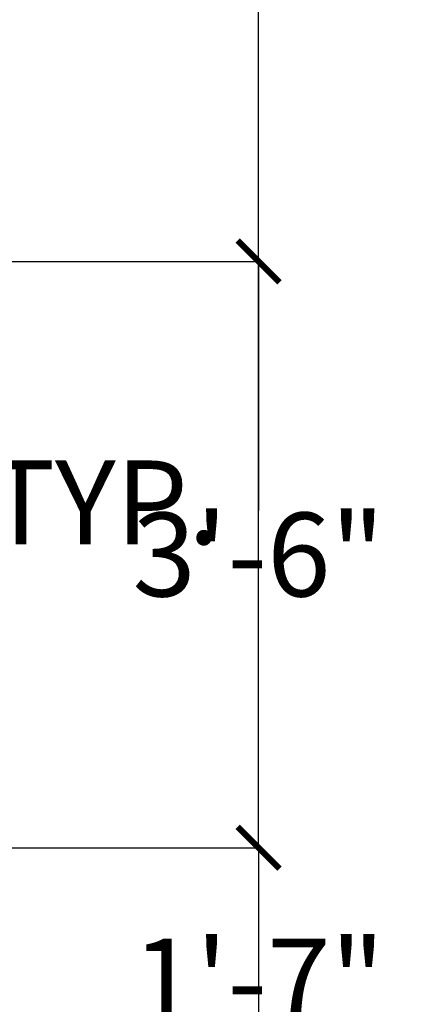
# Model space of a CAD drawing. Units: inches. Extents: x 2278 to 7495, y -71 to 1198.
# Tile 36 of 44: x 5150 to 5179, y 107 to 178. Entities that reach past the tile are written whole.
import ezdxf

# ---------------------------------------------------------------- set-up
doc = ezdxf.new("R2010")
doc.units = ezdxf.units.IN
doc.header["$MEASUREMENT"] = 0
doc.layers.add('A-ANNO-DIMS', color=2, linetype='Continuous', lineweight=18)
doc.styles.get("Standard").update_dxf_attribs({"font": 'arial.ttf'})
doc.dimstyles.get("Standard").update_dxf_attribs({"dimtxt": 6, "dimasz": 3, "dimexe": 0.18, "dimexo": 0.0625, "dimgap": 0.09, "dimtad": 0, "dimtih": 1, "dimtoh": 1, "dimdec": 0, "dimzin": 0, "dimdsep": 46, "dimlunit": 3, "dimtxsty": 'Standard', "dimblk": 'ARCHTICK', "dimcen": 0.09, "dimadec": 0, "dimazin": 0, "dimtfac": 1, "dimtdec": 0, "dimtofl": 0, "dimtmove": 0, "dimatfit": 3, "dimfxl": 1, "dimtolj": 1, "dimtzin": 0, "dimarcsym": 0})

# ---------------------------------------------------------------- blocks, each defined once
blk = doc.blocks.new('_ArchTick')
at = {"color": 0, "linetype": 'ByBlock', "const_width": 0.15}
blk.add_lwpolyline([(-0.5, -0.5), (0.5, 0.5)], dxfattribs=at)
blk = doc.blocks.new('*D59')
at = {"layer": 'A-ANNO-DIMS', "color": 0, "lineweight": -2, "transparency": 16777216}
for p, q in [((5096.589, 159.183), (5101.564, 159.183)), ((5101.384, 159.183), (5101.384, 146.185)), ((5101.384, 126.799), (5101.384, 139.796)), ((5096.589, 126.799), (5101.564, 126.799))]:
    blk.add_line(p, q, dxfattribs=at)
at = {"layer": 'Defpoints', "color": 0, "transparency": 16777216}
for p in [(5096.527, 159.183), (5101.384, 159.183), (5096.527, 126.799)]:
    blk.add_point(p, dxfattribs=at)
at = {"layer": 'A-ANNO-DIMS', "color": 0, "lineweight": -2, "transparency": 16777216, "xscale": 3, "yscale": 3, "zscale": 3}
for p, rotation in [((5101.384, 159.183), 90), ((5101.384, 126.799), 270)]:
    blk.add_blockref('_ArchTick', p, dxfattribs=dict(at, rotation=rotation))
at = {"layer": 'A-ANNO-DIMS', "color": 0, "transparency": 16777216, "insert": (5101.384, 142.991), "char_height": 6, "attachment_point": 5}
blk.add_mtext('\\A1;ORNATE BALUSTER 2\'-8 1/2" TYP.', dxfattribs=at)
blk = doc.blocks.new('*D138')
at = {"layer": 'A-ANNO-DIMS', "color": 0, "lineweight": -2, "transparency": 16777216}
for p, q in [((5145.739, 118.253), (5167.754, 118.253)), ((5167.574, 118.253), (5167.574, 111.855)), ((5167.574, 99.253), (5167.574, 105.651)), ((5096.239, 99.253), (5167.754, 99.253))]:
    blk.add_line(p, q, dxfattribs=at)
at = {"layer": 'Defpoints', "color": 0, "transparency": 16777216}
for p in [(5145.676, 118.253), (5167.574, 118.253), (5096.176, 99.253)]:
    blk.add_point(p, dxfattribs=at)
at = {"layer": 'A-ANNO-DIMS', "color": 0, "lineweight": -2, "transparency": 16777216, "xscale": 3, "yscale": 3, "zscale": 3}
for p, rotation in [((5167.574, 118.253), 90), ((5167.574, 99.253), 270)]:
    blk.add_blockref('_ArchTick', p, dxfattribs=dict(at, rotation=rotation))
at = {"layer": 'A-ANNO-DIMS', "color": 0, "transparency": 16777216, "insert": (5167.574, 108.753), "char_height": 6, "attachment_point": 5}
blk.add_mtext('\\A1;1\'-7"', dxfattribs=at)
blk = doc.blocks.new('*D139')
at = {"layer": 'A-ANNO-DIMS', "color": 0, "lineweight": -2, "transparency": 16777216}
for p, q in [((5092.239, 160.253), (5167.754, 160.253)), ((5167.574, 160.253), (5167.574, 142.408)), ((5167.574, 118.253), (5167.574, 136.097)), ((5145.739, 118.253), (5167.754, 118.253))]:
    blk.add_line(p, q, dxfattribs=at)
at = {"layer": 'Defpoints', "color": 0, "transparency": 16777216}
for p in [(5092.176, 160.253), (5167.574, 160.253), (5145.676, 118.253)]:
    blk.add_point(p, dxfattribs=at)
at = {"layer": 'A-ANNO-DIMS', "color": 0, "lineweight": -2, "transparency": 16777216, "xscale": 3, "yscale": 3, "zscale": 3}
for p, rotation in [((5167.574, 160.253), 90), ((5167.574, 118.253), 270)]:
    blk.add_blockref('_ArchTick', p, dxfattribs=dict(at, rotation=rotation))
at = {"layer": 'A-ANNO-DIMS', "color": 0, "transparency": 16777216, "insert": (5167.574, 139.253), "char_height": 6, "attachment_point": 5}
blk.add_mtext('\\A1;3\'-6"', dxfattribs=at)
blk = doc.blocks.new('*D140')
at = {"layer": 'A-ANNO-DIMS', "color": 0, "lineweight": -2, "transparency": 16777216}
for p, q in [((5096.239, 225.253), (5167.754, 225.253)), ((5167.574, 225.253), (5167.574, 195.894)), ((5167.574, 160.253), (5167.574, 189.612)), ((5092.239, 160.253), (5167.754, 160.253))]:
    blk.add_line(p, q, dxfattribs=at)
at = {"layer": 'Defpoints', "color": 0, "transparency": 16777216}
for p in [(5096.176, 225.253), (5167.574, 225.253), (5092.176, 160.253)]:
    blk.add_point(p, dxfattribs=at)
at = {"layer": 'A-ANNO-DIMS', "color": 0, "lineweight": -2, "transparency": 16777216, "xscale": 3, "yscale": 3, "zscale": 3}
for p, rotation in [((5167.574, 225.253), 90), ((5167.574, 160.253), 270)]:
    blk.add_blockref('_ArchTick', p, dxfattribs=dict(at, rotation=rotation))
at = {"layer": 'A-ANNO-DIMS', "color": 0, "transparency": 16777216, "insert": (5167.574, 192.753), "char_height": 6, "attachment_point": 5}
blk.add_mtext('\\A1;5\'-5"', dxfattribs=at)
blk = doc.blocks.new('*D143')
at = {"layer": 'A-ANNO-DIMS', "color": 0, "lineweight": -2, "transparency": 16777216}
for p, q in [((5145.739, 118.253), (5167.754, 118.253)), ((5167.574, 118.253), (5167.574, 61.406)), ((5167.574, -1.747), (5167.574, 55.099)), ((5145.739, -1.747), (5167.754, -1.747))]:
    blk.add_line(p, q, dxfattribs=at)
at = {"layer": 'Defpoints', "color": 0, "transparency": 16777216}
for p in [(5145.676, 118.253), (5167.574, 118.253), (5145.676, -1.747)]:
    blk.add_point(p, dxfattribs=at)
at = {"layer": 'A-ANNO-DIMS', "color": 0, "lineweight": -2, "transparency": 16777216, "xscale": 3, "yscale": 3, "zscale": 3}
for p, rotation in [((5167.574, 118.253), 90), ((5167.574, -1.747), 270)]:
    blk.add_blockref('_ArchTick', p, dxfattribs=dict(at, rotation=rotation))
at = {"layer": 'A-ANNO-DIMS', "color": 0, "transparency": 16777216, "insert": (5167.574, 58.253), "char_height": 6, "attachment_point": 5}
blk.add_mtext('\\A1;10\'-0"', dxfattribs=at)
blk = doc.blocks.new('*D144')
at = {"layer": 'A-ANNO-DIMS', "color": 0, "lineweight": -2, "transparency": 16777216}
for p, q in [((5145.739, 244.253), (5167.754, 244.253)), ((5167.574, 244.253), (5167.574, 184.406)), ((5167.574, 118.253), (5167.574, 178.099)), ((5145.739, 118.253), (5167.754, 118.253))]:
    blk.add_line(p, q, dxfattribs=at)
at = {"layer": 'Defpoints', "color": 0, "transparency": 16777216}
for p in [(5145.676, 244.253), (5167.574, 244.253), (5145.676, 118.253)]:
    blk.add_point(p, dxfattribs=at)
at = {"layer": 'A-ANNO-DIMS', "color": 0, "lineweight": -2, "transparency": 16777216, "xscale": 3, "yscale": 3, "zscale": 3}
for p, rotation in [((5167.574, 244.253), 90), ((5167.574, 118.253), 270)]:
    blk.add_blockref('_ArchTick', p, dxfattribs=dict(at, rotation=rotation))
at = {"layer": 'A-ANNO-DIMS', "color": 0, "transparency": 16777216, "insert": (5167.574, 181.253), "char_height": 6, "attachment_point": 5}
blk.add_mtext('\\A1;10\'-6"', dxfattribs=at)

msp = doc.modelspace()

# ---------------------------------------------------------------- dimensions: what is measured, and where the dimension line sits
at = {"layer": 'A-ANNO-DIMS'}
for base, p1, p2, picture, middle in [((5167.574, 244.253), (5145.676, 118.253), (5145.676, 244.253), '*D144', (5167.574, 181.253)), ((5167.574, 225.253), (5092.176, 160.253), (5096.176, 225.253), '*D140', (5167.574, 192.753)), ((5167.574, 160.253), (5145.676, 118.253), (5092.176, 160.253), '*D139', (5167.574, 139.253)), ((5167.574, 118.253), (5096.176, 99.253), (5145.676, 118.253), '*D138', (5167.574, 108.753)), ((5167.574, 118.253), (5145.676, -1.747), (5145.676, 118.253), '*D143', (5167.574, 58.253))]:
    dim = msp.add_linear_dim(base=base, p1=p1, p2=p2, angle=90, dimstyle='Standard', override={"dimdec": 1, "dimlfac": 1, "dimrnd": 0, "dimzin": 1, "dimdsep": 46, "dimlunit": 4, "dimfrac": 2}, dxfattribs=at)
    dim.commit()
    dim.dimension.update_dxf_attribs({"geometry": picture, "text_midpoint": middle})
dim = msp.add_linear_dim(base=(5101.384, 159.183), p1=(5096.527, 126.799), p2=(5096.527, 159.183), angle=90, text='ORNATE BALUSTER <> TYP.', dimstyle='Standard', override={"dimdec": 1, "dimrnd": 0, "dimzin": 1, "dimlunit": 4, "dimfrac": 2}, dxfattribs=at)
dim.commit()
dim.dimension.update_dxf_attribs({"geometry": '*D59', "text_midpoint": (5101.384, 142.991)})

doc.saveas('drawing.dxf')
